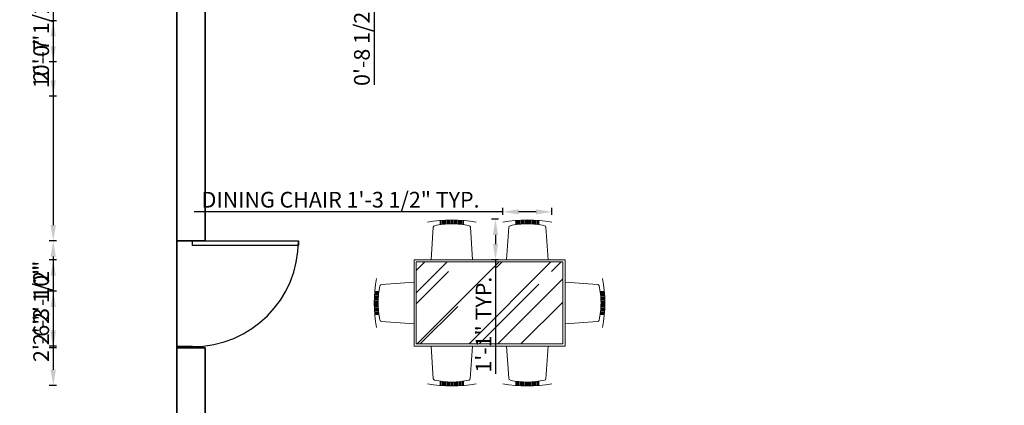
# Model space of a CAD drawing. Units: inches. Extents: x -48 to 817, y -530 to 78.
# Tile 2 of 7: x -48 to 266, y -276 to -153. Entities that reach past the tile are written whole.
import ezdxf

# ---------------------------------------------------------------- set-up
doc = ezdxf.new("R2010")
doc.units = ezdxf.units.IN
for name, color, linetype, lineweight in [('A-ANNO-DIMS', 2, 'Continuous', 18), ('A-DOOR', 3, 'Continuous', 25), ('A-FURN-PATT', 252, 'Continuous', 13), ('A-WALL', 7, 'Continuous', 35), ('furn', 8, 'Continuous', 18)]:
    doc.layers.add(name, color=color, linetype=linetype, lineweight=lineweight)
doc.styles.get("Standard").update_dxf_attribs({"font": 'arial.ttf'})
doc.dimstyles.new('ISO-25', dxfattribs={"dimtxt": 5, "dimasz": 5, "dimexe": 1.25, "dimexo": 0.625, "dimtad": 1, "dimlunit": 3, "dimtxsty": 'Standard', "dimcen": 2.5, "dimadec": 0, "dimazin": 0, "dimtfac": 1, "dimtmove": 0, "dimatfit": 3, "dimfxl": 1, "dimfxlon": 1, "dimarcsym": 0})

# ---------------------------------------------------------------- blocks, each defined once
blk = doc.blocks.new('*U2')
for p, q in [((0, 0), (0, -6)), ((40, 0), (40, -6))]:
    blk.add_line(p, q)
blk.add_lwpolyline([(0, 0), (0, 40), (1.75, 40), (1.75, 0)], close=True)
blk.add_arc((0, 0), 40, 0, 90)
blk = doc.blocks.new('CHAIR-DINING')
for p, q in [((1.19, 12.68), (1.89, 2.3)), ((14.38, 12.68), (13.67, 2.3)), ((4.1, 1.51), (4.1, 0.16)), ((4.44, 1.46), (4.44, 0.13)), ((4.78, 1.42), (4.78, 0.1)), ((5.13, 1.38), (5.13, 0.08)), ((5.47, 1.34), (5.47, 0.06)), ((5.81, 1.31), (5.81, 0.05)), ((6.16, 1.28), (6.16, 0.03)), ((6.5, 1.26), (6.5, 0.02)), ((6.84, 1.24), (6.84, 0.01)), ((7.18, 1.23), (7.18, 0)), ((7.53, 1.22), (7.53, 0)), ((7.78, 1.21), (7.78, 0)), ((8.04, 1.22), (8.04, 0)), ((8.38, 1.23), (8.38, 0)), ((8.73, 1.24), (8.73, 0.01)), ((9.07, 1.26), (9.07, 0.02)), ((9.41, 1.28), (9.41, 0.03)), ((9.75, 1.31), (9.75, 0.05)), ((10.1, 1.34), (10.1, 0.06)), ((10.44, 1.38), (10.44, 0.08)), ((10.78, 1.42), (10.78, 0.1)), ((11.13, 1.46), (11.13, 0.13)), ((11.47, 1.51), (11.47, 0.16))]:
    blk.add_line(p, q)
blk.add_lwpolyline([(0, 0.71, 0.091245), (15.57, 0.71, 0.091245)], format="xyb")
for centre, radius, start, end in [((2.4, 2.34), 0.514, 183.8745, 258.0355), ((8.28, 30.06), 28.85, 258.0355, 269.0138), ((7.29, 30.06), 28.85, 270.9862, 281.9645), ((13.16, 2.34), 0.514, 281.9645, 356.1255)]:
    blk.add_arc(centre, radius, start, end)
blk = doc.blocks.new('*D18')
at = {"layer": 'A-ANNO-DIMS', "color": 0, "lineweight": -2, "transparency": 16777216}
for p, q in [((106.14, -215.06), (106.14, -212.81)), ((121.7, -215.06), (121.7, -212.81)), ((106.14, -214.06), (7.95, -214.06)), ((116.7, -214.06), (111.14, -214.06))]:
    blk.add_line(p, q, dxfattribs=at)
at = {"layer": 'A-ANNO-DIMS', "color": 0, "transparency": 16777216}
for points in [[(111.14, -213.23), (111.14, -214.89), (106.14, -214.06)], [(116.7, -213.23), (116.7, -214.89), (121.7, -214.06)]]:
    blk.add_solid(points, dxfattribs=at)
at = {"layer": 'Defpoints', "color": 0, "transparency": 16777216}
for p in [(106.14, -214.06), (106.14, -216.39), (121.7, -216.39)]:
    blk.add_point(p, dxfattribs=at)
at = {"layer": 'A-ANNO-DIMS', "color": 0, "transparency": 16777216, "insert": (54.54, -210.85), "char_height": 5, "attachment_point": 5}
blk.add_mtext('DINING CHAIR 1\'-3 1/2" TYP.', dxfattribs=at)
blk = doc.blocks.new('*D19')
at = {"layer": 'A-ANNO-DIMS', "color": 0, "lineweight": -2, "transparency": 16777216}
for p, q in [((104.8, -216.39), (102.55, -216.39)), ((103.8, -221.39), (103.8, -224.31)), ((104.8, -229.31), (102.55, -229.31)), ((103.8, -229.31), (103.8, -265.57))]:
    blk.add_line(p, q, dxfattribs=at)
at = {"layer": 'A-ANNO-DIMS', "color": 0, "transparency": 16777216}
for points in [[(102.97, -221.39), (104.64, -221.39), (103.8, -216.39)], [(102.97, -224.31), (104.64, -224.31), (103.8, -229.31)]]:
    blk.add_solid(points, dxfattribs=at)
at = {"layer": 'Defpoints', "color": 0, "transparency": 16777216}
for p in [(106.14, -216.39), (103.8, -229.31), (106.14, -229.31)]:
    blk.add_point(p, dxfattribs=at)
at = {"layer": 'A-ANNO-DIMS', "color": 0, "transparency": 16777216, "insert": (100.67, -249.94), "char_height": 5, "attachment_point": 5, "rotation": 90}
blk.add_mtext('1\'-1" TYP.', dxfattribs=at)
blk = doc.blocks.new('*D41')
at = {"layer": 'A-ANNO-DIMS', "color": 0, "lineweight": -2, "transparency": 16777216}
for p, q in [((65.17, -124.02), (65.17, -119.02)), ((66.17, -129.02), (63.92, -129.02)), ((65.17, -129.02), (65.17, -137.52)), ((66.17, -137.52), (63.92, -137.52)), ((65.17, -142.52), (65.17, -173.71))]:
    blk.add_line(p, q, dxfattribs=at)
at = {"layer": 'A-ANNO-DIMS', "color": 0, "transparency": 16777216}
for points in [[(64.34, -124.02), (66.01, -124.02), (65.17, -129.02)], [(64.34, -142.52), (66.01, -142.52), (65.17, -137.52)]]:
    blk.add_solid(points, dxfattribs=at)
at = {"layer": 'Defpoints', "color": 0, "transparency": 16777216}
for p in [(66.97, -129.02), (65.17, -137.52), (66.97, -137.52)]:
    blk.add_point(p, dxfattribs=at)
at = {"layer": 'A-ANNO-DIMS', "color": 0, "transparency": 16777216, "insert": (61.96, -160.61), "char_height": 5, "attachment_point": 5, "rotation": 90}
blk.add_mtext('0\'-8 1/2"', dxfattribs=at)
blk = doc.blocks.new('*D46')
at = {"layer": 'A-ANNO-DIMS', "color": 0, "lineweight": -2, "transparency": 16777216}
for p, q in [((-35.87, -223.28), (-38.12, -223.28)), ((-36.87, -228.28), (-36.87, -252.28)), ((-35.87, -257.28), (-38.12, -257.28))]:
    blk.add_line(p, q, dxfattribs=at)
at = {"layer": 'A-ANNO-DIMS', "color": 0, "transparency": 16777216}
for points in [[(-37.71, -228.28), (-36.04, -228.28), (-36.87, -223.28)], [(-37.71, -252.28), (-36.04, -252.28), (-36.87, -257.28)]]:
    blk.add_solid(points, dxfattribs=at)
at = {"layer": 'Defpoints', "color": 0, "transparency": 16777216}
for p in [(2.43, -223.28), (-36.87, -257.28), (2.43, -257.28)]:
    blk.add_point(p, dxfattribs=at)
at = {"layer": 'A-ANNO-DIMS', "color": 0, "transparency": 16777216, "insert": (-40.05, -240.28), "char_height": 5, "attachment_point": 5, "rotation": 90}
blk.add_mtext('2\'-10"', dxfattribs=at)
blk = doc.blocks.new('*D51')
at = {"layer": 'A-ANNO-DIMS', "color": 0, "lineweight": -2, "transparency": 16777216}
for p, q in [((-35.87, -95.58), (-38.12, -95.58)), ((-36.87, -100.58), (-36.87, -218.28)), ((-35.87, -223.28), (-38.12, -223.28))]:
    blk.add_line(p, q, dxfattribs=at)
at = {"layer": 'A-ANNO-DIMS', "color": 0, "transparency": 16777216}
for points in [[(-37.71, -100.58), (-36.04, -100.58), (-36.87, -95.58)], [(-37.71, -218.28), (-36.04, -218.28), (-36.87, -223.28)]]:
    blk.add_solid(points, dxfattribs=at)
at = {"layer": 'Defpoints', "color": 0, "transparency": 16777216}
for p in [(2.43, -95.58), (-36.87, -223.28), (2.43, -223.28)]:
    blk.add_point(p, dxfattribs=at)
at = {"layer": 'A-ANNO-DIMS', "color": 0, "transparency": 16777216, "insert": (-40.08, -159.43), "char_height": 5, "attachment_point": 5, "rotation": 90}
blk.add_mtext('10\'-7 1/2"', dxfattribs=at)
blk = doc.blocks.new('*D59')
at = {"layer": 'A-ANNO-DIMS', "color": 0, "lineweight": -2, "transparency": 16777216}
for p, q in [((155.43, -506.59), (155.43, -508.84)), ((161.43, -506.59), (161.43, -508.84)), ((150.43, -507.59), (145.43, -507.59)), ((155.43, -507.59), (161.43, -507.59)), ((166.43, -507.59), (185.97, -507.59))]:
    blk.add_line(p, q, dxfattribs=at)
at = {"layer": 'A-ANNO-DIMS', "color": 0, "transparency": 16777216}
for points in [[(150.43, -506.76), (150.43, -508.42), (155.43, -507.59)], [(166.43, -506.76), (166.43, -508.42), (161.43, -507.59)]]:
    blk.add_solid(points, dxfattribs=at)
at = {"layer": 'Defpoints', "color": 0, "transparency": 16777216}
for p in [(155.43, -141.28), (161.43, -147.28), (161.43, -507.59)]:
    blk.add_point(p, dxfattribs=at)
at = {"layer": 'A-ANNO-DIMS', "color": 0, "transparency": 16777216, "insert": (178.7, -504.41), "char_height": 5, "attachment_point": 5}
blk.add_mtext('0\'-6"', dxfattribs=at)
blk = doc.blocks.new('*D62')
at = {"layer": 'A-ANNO-DIMS', "color": 0, "lineweight": -2, "transparency": 16777216}
for p, q in [((-35.87, -239.28), (-38.12, -239.28)), ((-36.87, -244.28), (-36.87, -264.28)), ((-35.87, -269.28), (-38.12, -269.28))]:
    blk.add_line(p, q, dxfattribs=at)
at = {"layer": 'A-ANNO-DIMS', "color": 0, "transparency": 16777216}
for points in [[(-37.71, -244.28), (-36.04, -244.28), (-36.87, -239.28)], [(-37.71, -264.28), (-36.04, -264.28), (-36.87, -269.28)]]:
    blk.add_solid(points, dxfattribs=at)
at = {"layer": 'Defpoints', "color": 0, "transparency": 16777216}
for p in [(593.43, -239.28), (-36.87, -269.28), (593.43, -269.28)]:
    blk.add_point(p, dxfattribs=at)
at = {"layer": 'A-ANNO-DIMS', "color": 0, "transparency": 16777216, "insert": (-40.05, -254.28), "char_height": 5, "attachment_point": 5, "rotation": 90}
blk.add_mtext('2\'-6"', dxfattribs=at)
blk = doc.blocks.new('*D68')
at = {"layer": 'A-ANNO-DIMS', "color": 0, "lineweight": -2, "transparency": 16777216}
for p, q in [((-35.87, -153.28), (-38.12, -153.28)), ((-36.87, -158.28), (-36.87, -172.28)), ((-35.87, -177.28), (-38.12, -177.28))]:
    blk.add_line(p, q, dxfattribs=at)
at = {"layer": 'A-ANNO-DIMS', "color": 0, "transparency": 16777216}
for points in [[(-37.71, -158.28), (-36.04, -158.28), (-36.87, -153.28)], [(-37.71, -172.28), (-36.04, -172.28), (-36.87, -177.28)]]:
    blk.add_solid(points, dxfattribs=at)
at = {"layer": 'Defpoints', "color": 0, "transparency": 16777216}
for p in [(570.33, -153.28), (-36.87, -177.28), (570.33, -177.28)]:
    blk.add_point(p, dxfattribs=at)
at = {"layer": 'A-ANNO-DIMS', "color": 0, "transparency": 16777216, "insert": (-40.05, -165.28), "char_height": 5, "attachment_point": 5, "rotation": 90}
blk.add_mtext('2\'-0"', dxfattribs=at)
blk = doc.blocks.new('*D71')
at = {"layer": 'A-ANNO-DIMS', "color": 0, "lineweight": -2, "transparency": 16777216}
for p, q in [((11.43, -506.59), (11.43, -508.84)), ((101.43, -506.59), (101.43, -508.84)), ((16.43, -507.59), (96.43, -507.59))]:
    blk.add_line(p, q, dxfattribs=at)
at = {"layer": 'A-ANNO-DIMS', "color": 0, "transparency": 16777216}
for points in [[(16.43, -506.76), (16.43, -508.42), (11.43, -507.59)], [(96.43, -506.76), (96.43, -508.42), (101.43, -507.59)]]:
    blk.add_solid(points, dxfattribs=at)
at = {"layer": 'Defpoints', "color": 0, "transparency": 16777216}
for p in [(11.43, 2.72), (101.43, 2.72), (101.43, -507.59)]:
    blk.add_point(p, dxfattribs=at)
at = {"layer": 'A-ANNO-DIMS', "color": 0, "transparency": 16777216, "insert": (56.43, -504.41), "char_height": 5, "attachment_point": 5}
blk.add_mtext('7\'-6"', dxfattribs=at)
blk = doc.blocks.new('*D77')
at = {"layer": 'A-ANNO-DIMS', "color": 0, "lineweight": -2, "transparency": 16777216}
for p, q in [((77.91, -506.59), (77.91, -508.84)), ((125.92, -506.59), (125.92, -508.84)), ((82.91, -507.59), (120.92, -507.59))]:
    blk.add_line(p, q, dxfattribs=at)
at = {"layer": 'A-ANNO-DIMS', "color": 0, "transparency": 16777216}
for points in [[(82.91, -506.76), (82.91, -508.42), (77.91, -507.59)], [(120.92, -506.76), (120.92, -508.42), (125.92, -507.59)]]:
    blk.add_solid(points, dxfattribs=at)
at = {"layer": 'Defpoints', "color": 0, "transparency": 16777216}
for p in [(77.91, -256.74), (125.92, -256.74), (125.92, -507.59)]:
    blk.add_point(p, dxfattribs=at)
at = {"layer": 'A-ANNO-DIMS', "color": 0, "transparency": 16777216, "insert": (101.92, -504.41), "char_height": 5, "attachment_point": 5}
blk.add_mtext('4\'-0"', dxfattribs=at)
blk = doc.blocks.new('*D78')
at = {"layer": 'A-ANNO-DIMS', "color": 0, "lineweight": -2, "transparency": 16777216}
for p, q in [((-35.87, -229.31), (-38.12, -229.31)), ((-36.87, -234.31), (-36.87, -251.74)), ((-35.87, -256.74), (-38.12, -256.74))]:
    blk.add_line(p, q, dxfattribs=at)
at = {"layer": 'A-ANNO-DIMS', "color": 0, "transparency": 16777216}
for points in [[(-37.71, -234.31), (-36.04, -234.31), (-36.87, -229.31)], [(-37.71, -251.74), (-36.04, -251.74), (-36.87, -256.74)]]:
    blk.add_solid(points, dxfattribs=at)
at = {"layer": 'Defpoints', "color": 0, "transparency": 16777216}
for p in [(77.91, -229.31), (-36.87, -256.74), (77.91, -256.74)]:
    blk.add_point(p, dxfattribs=at)
at = {"layer": 'A-ANNO-DIMS', "color": 0, "transparency": 16777216, "insert": (-40.08, -243.03), "char_height": 5, "attachment_point": 5, "rotation": 90}
blk.add_mtext('2\'-3 1/2"', dxfattribs=at)
blk = doc.blocks.new('*D80')
at = {"layer": 'A-ANNO-DIMS', "color": 0, "lineweight": -2, "transparency": 16777216}
for p, q in [((-35.87, -63.95), (-38.12, -63.95)), ((-36.87, -68.95), (-36.87, -161.39)), ((-35.87, -166.39), (-38.12, -166.39))]:
    blk.add_line(p, q, dxfattribs=at)
at = {"layer": 'A-ANNO-DIMS', "color": 0, "transparency": 16777216}
for points in [[(-37.71, -68.95), (-36.04, -68.95), (-36.87, -63.95)], [(-37.71, -161.39), (-36.04, -161.39), (-36.87, -166.39)]]:
    blk.add_solid(points, dxfattribs=at)
at = {"layer": 'Defpoints', "color": 0, "transparency": 16777216}
for p in [(447.47, -63.95), (-36.87, -166.39), (447.47, -166.39)]:
    blk.add_point(p, dxfattribs=at)
at = {"layer": 'A-ANNO-DIMS', "color": 0, "transparency": 16777216, "insert": (-40.08, -115.17), "char_height": 5, "attachment_point": 5, "rotation": 90}
blk.add_mtext('8\'-6 1/2"', dxfattribs=at)

msp = doc.modelspace()

# ---------------------------------------------------------------- hatches: boundary and pattern name
at = {"layer": 'A-FURN-PATT'}
h = msp.add_hatch(dxfattribs=at)
h.set_pattern_fill('AR-RROOF', color=256, scale=0.685868, angle=45, style=0)
h.set_pattern_definition([(45, (-1181.963, -828.06), (14.78226, 39.41935), [261.3158, -34.8421, 87.1053, -17.421]), (45, (-1171.739, -805.517), (-28.7022, 4.06512), [52.2632, -5.749, 104.5263, -13.0658]), (45, (-1186.275, -811.43), (55.80302, 72.30987), [139.36845, -24.3895, 69.6842, -17.42106])])
h.paths.add_polyline_path([(78.599, -229.994), (78.599, -256.057), (125.238, -256.057), (125.238, -229.994)])

# ---------------------------------------------------------------- linework, layer by layer
at = {"layer": 'A-WALL'}
for p, q in [((2.427, -468.275), (2.427, 11.725)), ((11.427, -223.275), (11.427, 2.725)), ((11.427, -223.275), (2.427, -223.275)), ((11.427, -257.275), (2.427, -257.275)), ((11.427, -459.275), (11.427, -257.275))]:
    msp.add_line(p, q, dxfattribs=at)
at = {"layer": 'furn'}
for p, q in [((107.327, -256.743), (108.021, -266.99)), ((120.516, -256.743), (119.813, -267.119)), ((110.236, -267.91), (110.236, -269.263)), ((110.579, -267.958), (110.579, -269.291)), ((110.922, -268.002), (110.922, -269.316)), ((111.265, -268.042), (111.265, -269.339)), ((111.608, -268.078), (111.608, -269.359)), ((111.95, -268.109), (111.95, -269.376)), ((112.293, -268.136), (112.293, -269.39)), ((112.636, -268.16), (112.636, -269.402)), ((112.979, -268.179), (112.979, -269.411)), ((113.322, -268.194), (113.322, -269.417)), ((113.665, -268.205), (113.665, -269.42)), ((113.921, -268.21), (113.921, -269.421)), ((114.178, -268.205), (114.178, -269.42)), ((114.521, -268.194), (114.521, -269.417)), ((114.864, -268.179), (114.864, -269.411)), ((115.207, -268.16), (115.207, -269.402)), ((115.55, -268.136), (115.55, -269.39)), ((115.892, -268.109), (115.892, -269.376)), ((116.235, -268.078), (116.235, -269.359)), ((116.578, -268.042), (116.578, -269.339)), ((116.921, -268.002), (116.921, -269.316)), ((117.264, -267.958), (117.264, -269.291)), ((117.607, -267.91), (117.607, -269.263))]:
    msp.add_line(p, q, dxfattribs=at)
for points in [[(77.913, -256.743), (125.924, -256.743), (125.924, -229.308), (77.913, -229.308)], [(78.599, -256.057), (125.238, -256.057), (125.238, -229.994), (78.599, -229.994)]]:
    msp.add_lwpolyline(points, close=True, dxfattribs=at)
msp.add_lwpolyline([(121.704, -268.711, -0.0912453), (106.139, -268.711, -0.0912453)], format="xyb", dxfattribs=at)
for centre, radius, start, end in [((108.705, -266.944), 0.686, 183.87448, 258.29889), ((114.418, -239.361), 28.854, 258.29889, 269.01382), ((113.425, -239.361), 28.854, 270.98618, 281.96453), ((119.3, -267.085), 0.514, 281.96453, 356.12552)]:
    msp.add_arc(centre, radius, start, end, dxfattribs=at)

# ---------------------------------------------------------------- block references
at = {"layer": 'A-DOOR', "xscale": 0.841334761058589, "yscale": 0.841334761058589, "zscale": 0.841334761058589, "rotation": 270}
msp.add_blockref('*U2', (7.475, -223.275), dxfattribs=at)
at = {"layer": 'furn'}
for p, rotation in [((97.699, -216.63), 180), ((121.705, -216.63), 180), ((65.235, -235.243), 270.0000000039537), ((138.602, -250.809), 90.00000000367844)]:
    msp.add_blockref('CHAIR-DINING', p, dxfattribs=dict(at, rotation=rotation))
msp.add_blockref('CHAIR-DINING', (82.133, -269.421), dxfattribs=at)

# ---------------------------------------------------------------- dimensions: what is measured, and where the dimension line sits
at = {"layer": 'A-ANNO-DIMS'}
for base, p1, p2, picture, middle in [((101.427, -507.589), (11.427, 2.725), (101.427, 2.725), '*D71', (56.427, -504.411)), ((161.427, -507.589), (155.427, -141.275), (161.427, -147.275), '*D59', (178.698, -504.411)), ((125.924, -507.589), (77.913, -256.743), (125.924, -256.743), '*D77', (101.919, -504.411))]:
    dim = msp.add_linear_dim(base=base, p1=p1, p2=p2, dimstyle='ISO-25', override={"dimdec": 1, "dimlfac": 1, "dimrnd": 0, "dimzin": 1, "dimdsep": 46, "dimlunit": 4, "dimfrac": 2}, dxfattribs=at)
    dim.commit()
    dim.dimension.update_dxf_attribs({"geometry": picture, "text_midpoint": middle})
for base, p1, p2, angle, picture, middle in [((-36.873, -166.393), (447.473, -63.949), (447.473, -166.393), 90, '*D80', (-40.083, -115.171)), ((-36.873, -223.275), (2.427, -95.585), (2.427, -223.275), 90, '*D51', (-40.083, -159.43)), ((65.175, -137.519), (66.975, -129.02), (66.975, -137.519), 270, '*D41', (61.965, -160.615)), ((-36.873, -177.275), (570.327, -153.275), (570.327, -177.275), 90, '*D68', (-40.051, -165.275)), ((-36.873, -257.275), (2.427, -223.275), (2.427, -257.275), 90, '*D46', (-40.051, -240.275)), ((-36.873, -256.743), (77.913, -229.308), (77.913, -256.743), 90, '*D78', (-40.085, -243.026)), ((-36.873, -269.275), (593.427, -239.275), (593.427, -269.275), 90, '*D62', (-40.051, -254.275))]:
    dim = msp.add_linear_dim(base=base, p1=p1, p2=p2, angle=angle, dimstyle='ISO-25', override={"dimdec": 1, "dimlfac": 1, "dimrnd": 0, "dimzin": 1, "dimdsep": 46, "dimlunit": 4, "dimfrac": 2}, dxfattribs=at)
    dim.commit()
    dim.dimension.update_dxf_attribs({"geometry": picture, "text_midpoint": middle})
for base, p1, p2, angle, text, picture, middle in [((106.139, -214.059), (121.704, -216.394), (106.139, -216.394), 180, 'DINING CHAIR <> TYP.', '*D18', (54.543, -210.847)), ((103.804, -229.308), (106.139, -216.394), (106.139, -229.308), 270, '<> TYP.', '*D19', (100.667, -249.937))]:
    dim = msp.add_linear_dim(base=base, p1=p1, p2=p2, angle=angle, text=text, dimstyle='ISO-25', override={"dimdec": 1, "dimlfac": 1, "dimrnd": 0, "dimzin": 1, "dimdsep": 46, "dimlunit": 4, "dimfrac": 2}, dxfattribs=at)
    dim.commit()
    dim.dimension.update_dxf_attribs({"geometry": picture, "text_midpoint": middle})

doc.saveas('drawing.dxf')
